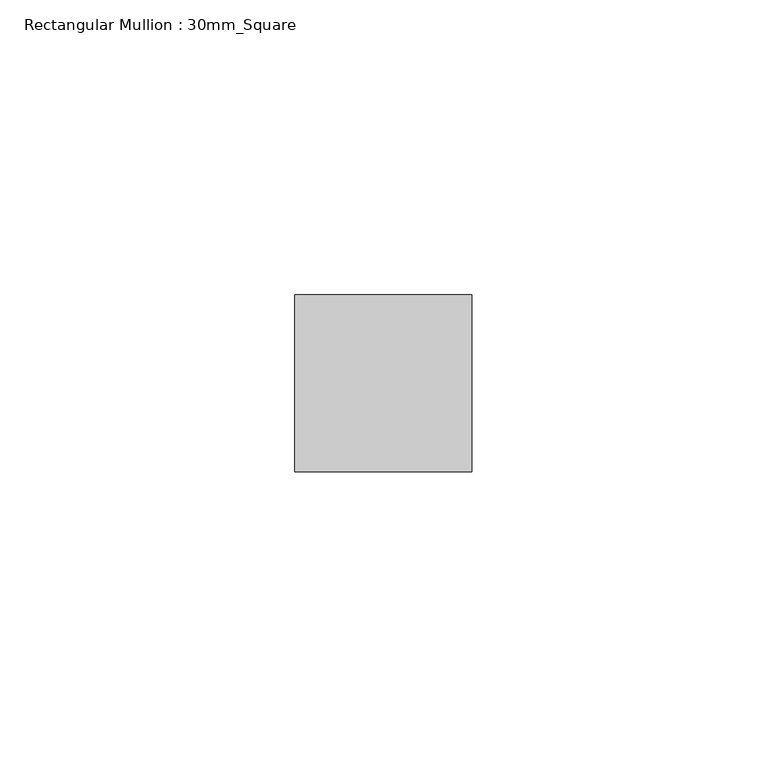
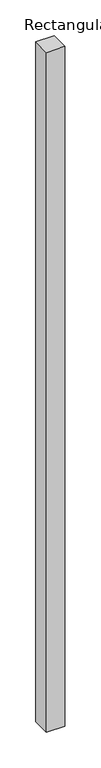
"""IFC4 building model written with IfcOpenShell, lengths in millimetres: member geometry, Rectangular Mullion : 30mm_Square."""

from ifc_helpers import new_model, si_unit, frame, origin, place, context, project, spatial, polyline, outline, extrude, source, transform, mapped, element, save


def rectangular_mullion_30mm_square_ea944ed7(model_context):
    return source(origin(), model_context, "Body", "SweptSolid", [
        extrude(outline(polyline([(0.0, 15.0), (0.0, -15.0), (-30.0, -15.0), (-30.0, 15.0), (0.0, 15.0)])), frame((0.0, 0.0, -1161.7008958), z_axis=(0.0, 0.0, 1.0), x_axis=(1.0, 0.0, 0.0)), (0.0, 0.0, 1.0), 1161.7008958),
    ])


if __name__ == "__main__":
    model = new_model("IFC4")
    model_context = context("Model", 3, world=origin())
    ifc_project = project(units=[si_unit("LENGTHUNIT", "METRE", prefix="MILLI")], contexts=[model_context])
    site = spatial("IfcSite", under=ifc_project)
    building = spatial("IfcBuilding", under=site)
    placement = place(None, origin())
    rectangular_mullion_30mm_square_shape = rectangular_mullion_30mm_square_ea944ed7(model_context)
    element("IfcMember", 1, ObjectType="Rectangular Mullion : 30mm_Square", at=placement, inside=building, context=model_context, shape_type="MappedRepresentation", body=[
        mapped(rectangular_mullion_30mm_square_shape, transform((0.0, 0.0, 0.0), x_axis=(1.0, 0.0, 0.0), y_axis=(0.0, 1.0, 0.0), z_axis=(0.0, 0.0, 1.0))),
    ])
    save(model, "model.ifc")

# Revit data of these elements
# Type "Rectangular Mullion : 30mm_Square"
#   Keynote = "H11"
#   built-in parameter 1007304 = 0.0984252 (stored number, unit not read)
#   built-in parameter 1007301 = 0.0492126 (stored number, unit not read)
#   built-in parameter 1007300 = 0.0492126 (stored number, unit not read)
# Element 1 (IfcMember, "Rectangular Mullion : 30mm_Square")
#   Materials on its faces: "Aluminium"
# Materials
#   "Aluminium": class "Metal", colour RGB 247 247 247, transparency 0, Description = "Aluminium 6061", Cost = 0
